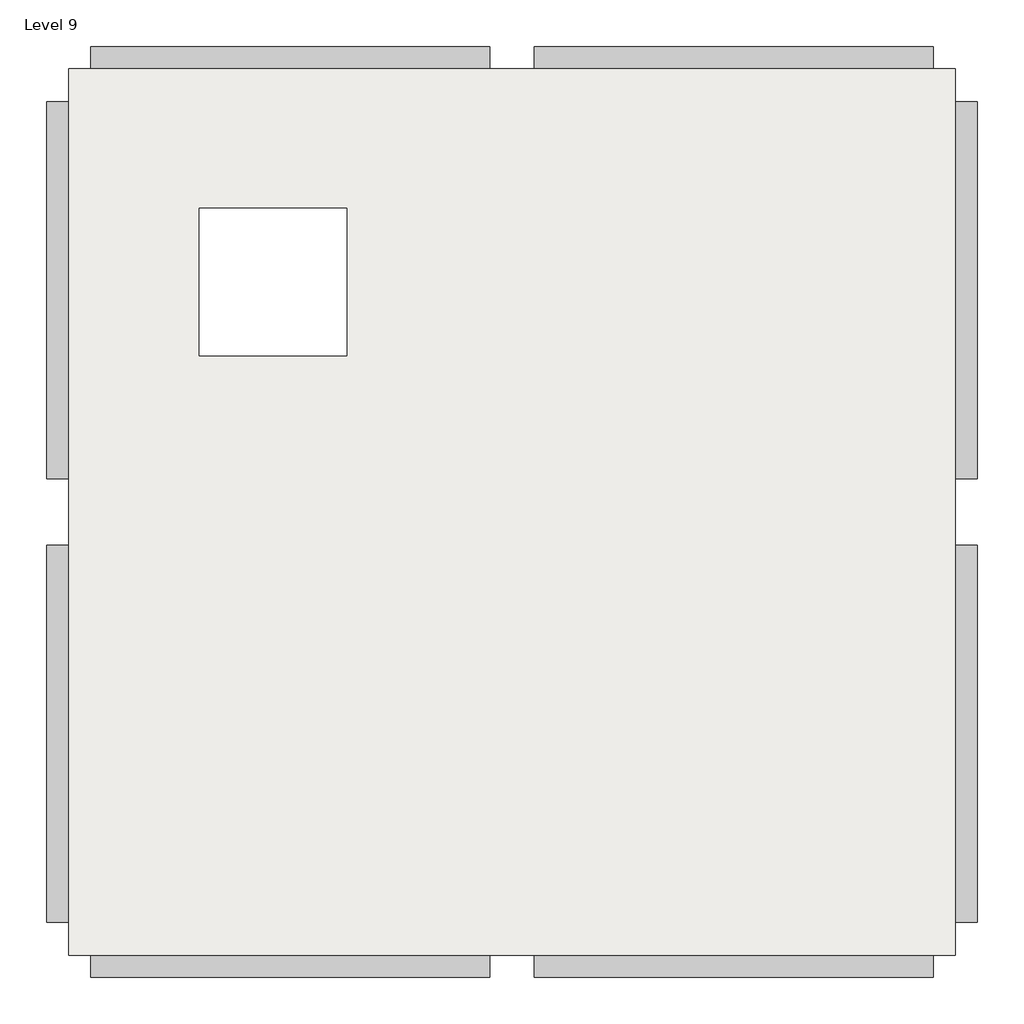
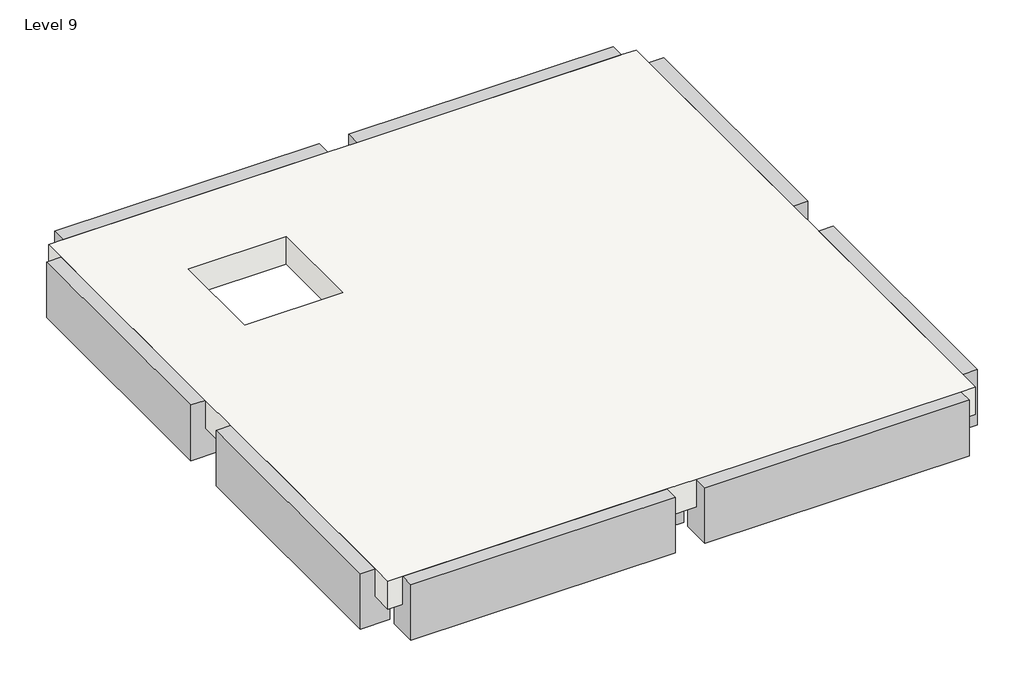
# One storey: 6 beams, 1 slab.
"""IFC4 building model written with IfcOpenShell, lengths in millimetres."""

from ifc_helpers import new_model, si_unit, frame, origin, place, context, project, spatial, polyline, outline, extrude, faceted_brep, element, save

model = new_model("IFC4")

# Units and contexts
model_context = context("Model", 3, world=origin())
ifc_project = project(units=[si_unit("LENGTHUNIT", "METRE", prefix="MILLI")], contexts=[model_context])

# Site, building, storey
site = spatial("IfcSite", under=ifc_project)
building = spatial("IfcBuilding", under=site)
storey = spatial("IfcBuildingStorey", under=building, Name="Level 9", Elevation=24000.0)

# Beams
placement = place(None, origin())
element("IfcBeam", 1, ObjectType="Concrete-Rectangular Beam : 300 x 600mm", at=placement, inside=storey, context=model_context, shape_type="SweptSolid", body=[
    extrude(outline(polyline([(526.3372902, 23400.0), (226.3372902, 23400.0), (226.3372902, 23700.0), (376.3372902, 23700.0), (376.3372902, 24000.0), (526.3372902, 24000.0), (526.3372902, 23400.0)])), frame((2068.7595868, 0.0, 0.0), z_axis=(1.0, 0.0, 0.0), x_axis=(0.0, 1.0, 0.0)), (0.0, 0.0, 1.0), 2700.0),
    extrude(outline(polyline([(526.3372902, 23400.0), (226.3372902, 23400.0), (226.3372902, 23700.0), (376.3372902, 23700.0), (376.3372902, 24000.0), (526.3372902, 24000.0), (526.3372902, 23400.0)])), frame((-931.2404132, 0.0, 0.0), z_axis=(1.0, 0.0, 0.0), x_axis=(0.0, 1.0, 0.0)), (0.0, 0.0, 1.0), 2700.0),
])
element("IfcBeam", 2, ObjectType="Concrete-Rectangular Beam : 300 x 600mm", at=placement, inside=storey, context=model_context, shape_type="SweptSolid", body=[
    extrude(outline(polyline([(23400.0, 5068.7595868), (24000.0, 5068.7595868), (24000.0, 4918.7595868), (23700.0, 4918.7595868), (23700.0, 4768.7595868), (23400.0, 4768.7595868), (23400.0, 5068.7595868)])), frame((0.0, -2398.6627098, 0.0), z_axis=(0.0, 1.0, 0.0), x_axis=(0.0, 0.0, 1.0)), (0.0, 0.0, 1.0), 2550.0),
    extrude(outline(polyline([(23400.0, 5068.7595868), (24000.0, 5068.7595868), (24000.0, 4918.7595868), (23700.0, 4918.7595868), (23700.0, 4768.7595868), (23400.0, 4768.7595868), (23400.0, 5068.7595868)])), frame((0.0, -5398.6627098, 0.0), z_axis=(0.0, 1.0, 0.0), x_axis=(0.0, 0.0, 1.0)), (0.0, 0.0, 1.0), 2550.0),
])
element("IfcBeam", 3, ObjectType="Concrete-Rectangular Beam : 300 x 600mm", at=placement, inside=storey, context=model_context, shape_type="SweptSolid", body=[
    extrude(outline(polyline([(-5773.6627098, 23400.0), (-5773.6627098, 24000.0), (-5623.6627098, 24000.0), (-5623.6627098, 23700.0), (-5473.6627098, 23700.0), (-5473.6627098, 23400.0), (-5773.6627098, 23400.0)])), frame((2068.7595868, 0.0, 0.0), z_axis=(1.0, 0.0, 0.0), x_axis=(0.0, 1.0, 0.0)), (0.0, 0.0, 1.0), 2700.0),
    extrude(outline(polyline([(-5773.6627098, 23400.0), (-5773.6627098, 24000.0), (-5623.6627098, 24000.0), (-5623.6627098, 23700.0), (-5473.6627098, 23700.0), (-5473.6627098, 23400.0), (-5773.6627098, 23400.0)])), frame((-931.2404132, 0.0, 0.0), z_axis=(1.0, 0.0, 0.0), x_axis=(0.0, 1.0, 0.0)), (0.0, 0.0, 1.0), 2700.0),
])
element("IfcBeam", 4, ObjectType="Concrete-Rectangular Beam : 300 x 600mm", at=placement, inside=storey, context=model_context, shape_type="SweptSolid", body=[
    extrude(outline(polyline([(24000.0, -1231.2404132), (23400.0, -1231.2404132), (23400.0, -931.2404132), (23700.0, -931.2404132), (23700.0, -1081.2404132), (24000.0, -1081.2404132), (24000.0, -1231.2404132)])), frame((0.0, -5398.6627098, 0.0), z_axis=(0.0, 1.0, 0.0), x_axis=(0.0, 0.0, 1.0)), (0.0, 0.0, 1.0), 2550.0),
    extrude(outline(polyline([(24000.0, -1231.2404132), (23400.0, -1231.2404132), (23400.0, -931.2404132), (23700.0, -931.2404132), (23700.0, -1081.2404132), (24000.0, -1081.2404132), (24000.0, -1231.2404132)])), frame((0.0, -2398.6627098, 0.0), z_axis=(0.0, 1.0, 0.0), x_axis=(0.0, 0.0, 1.0)), (0.0, 0.0, 1.0), 2550.0),
])
element("IfcBeam", 5, ObjectType="Concrete-Rectangular Beam : 300 x 600mm", at=placement, inside=storey, context=model_context, shape_type="SweptSolid", body=[
    extrude(outline(polyline([(2068.7595868, -5398.6627098), (1768.7595868, -5398.6627098), (1768.7595868, -2848.6627098), (2068.7595868, -2848.6627098), (2068.7595868, -5398.6627098)])), frame((0.0, 0.0, 23400.0), z_axis=(0.0, 0.0, 1.0), x_axis=(1.0, 0.0, 0.0)), (0.0, 0.0, 1.0), 300.0),
    extrude(outline(polyline([(1768.7595868, 151.3372902), (2068.7595868, 151.3372902), (2068.7595868, -2398.6627098), (1768.7595868, -2398.6627098), (1768.7595868, 151.3372902)])), frame((0.0, 0.0, 23400.0), z_axis=(0.0, 0.0, 1.0), x_axis=(1.0, 0.0, 0.0)), (0.0, 0.0, 1.0), 300.0),
])
element("IfcBeam", 6, ObjectType="Concrete-Rectangular Beam : 300 x 600mm", at=placement, inside=storey, context=model_context, shape_type="SweptSolid", body=[
    extrude(outline(polyline([(4768.7595868, -2473.6627098), (4768.7595868, -2773.6627098), (2068.7595868, -2773.6627098), (2068.7595868, -2473.6627098), (4768.7595868, -2473.6627098)])), frame((0.0, 0.0, 23400.0), z_axis=(0.0, 0.0, 1.0), x_axis=(1.0, 0.0, 0.0)), (0.0, 0.0, 1.0), 300.0),
    extrude(outline(polyline([(-931.2404132, -2773.6627098), (-931.2404132, -2473.6627098), (1768.7595868, -2473.6627098), (1768.7595868, -2773.6627098), (-931.2404132, -2773.6627098)])), frame((0.0, 0.0, 23400.0), z_axis=(0.0, 0.0, 1.0), x_axis=(1.0, 0.0, 0.0)), (0.0, 0.0, 1.0), 300.0),
])

# Slab
element("IfcSlab", 7, ObjectType="Generic 300mm", at=placement, inside=storey, context=model_context, shape_type="Brep", body=[
    faceted_brep([(4918.7595868, 376.3372902, 23700.0), (4918.7595868, 151.3372902, 23700.0), (4918.7595868, -2398.6627098, 23700.0), (4918.7595868, -2848.6627098, 23700.0), (4918.7595868, -5398.6627098, 23700.0), (4918.7595868, -5623.6627098, 23700.0), (4768.7595868, -5623.6627098, 23700.0), (2068.7595868, -5623.6627098, 23700.0), (1768.7595868, -5623.6627098, 23700.0), (-931.2404132, -5623.6627098, 23700.0), (-1081.2404132, -5623.6627098, 23700.0), (-1081.2404132, -5398.6627098, 23700.0), (-1081.2404132, -2848.6627098, 23700.0), (-1081.2404132, -2398.6627098, 23700.0), (-1081.2404132, 151.3372902, 23700.0), (-1081.2404132, 376.3372902, 23700.0), (-931.2404132, 376.3372902, 23700.0), (1768.7595868, 376.3372902, 23700.0), (2068.7595868, 376.3372902, 23700.0), (4768.7595868, 376.3372902, 23700.0), (-198.5229478, -1566.5574371, 23700.0), (801.4770522, -1566.5574371, 23700.0), (801.4770522, -566.5574371, 23700.0), (-198.5229478, -566.5574371, 23700.0), (4918.7595868, -5623.6627098, 24000.0), (4918.7595868, -5398.6627098, 24000.0), (4918.7595868, -2848.6627098, 24000.0), (4918.7595868, -2398.6627098, 24000.0), (4918.7595868, 151.3372902, 24000.0), (4918.7595868, 376.3372902, 24000.0), (4768.7595868, 376.3372902, 24000.0), (2068.7595868, 376.3372902, 24000.0), (1768.7595868, 376.3372902, 24000.0), (-931.2404132, 376.3372902, 24000.0), (-1081.2404132, 376.3372902, 24000.0), (-1081.2404132, 151.3372902, 24000.0), (-1081.2404132, -2398.6627098, 24000.0), (-1081.2404132, -2848.6627098, 24000.0), (-1081.2404132, -5398.6627098, 24000.0), (-1081.2404132, -5623.6627098, 24000.0), (-931.2404132, -5623.6627098, 24000.0), (1768.7595868, -5623.6627098, 24000.0), (2068.7595868, -5623.6627098, 24000.0), (4768.7595868, -5623.6627098, 24000.0), (801.4770522, -1566.5574371, 24000.0), (-198.5229478, -1566.5574371, 24000.0), (-198.5229478, -566.5574371, 24000.0), (801.4770522, -566.5574371, 24000.0)], [[[0, 1, 2, 3, 4, 5, 6, 7, 8, 9, 10, 11, 12, 13, 14, 15, 16, 17, 18, 19], [20, 21, 22, 23]], [[24, 25, 26, 27, 28, 29, 30, 31, 32, 33, 34, 35, 36, 37, 38, 39, 40, 41, 42, 43], [44, 45, 46, 47]], [[5, 4, 3, 2, 1, 0, 29, 28, 27, 26, 25, 24]], [[10, 9, 8, 7, 6, 5, 24, 43, 42, 41, 40, 39]], [[15, 14, 13, 12, 11, 10, 39, 38, 37, 36, 35, 34]], [[0, 19, 18, 17, 16, 15, 34, 33, 32, 31, 30, 29]], [[20, 45, 44, 21]], [[21, 44, 47, 22]], [[22, 47, 46, 23]], [[45, 20, 23, 46]]]),
])

save(model, "model.ifc")

# Revit data of these elements
# Type "Concrete-Rectangular Beam : 300 x 600mm"
#   Length [instance default] = 1.524 m
#   b = 0.3 m
#   h = 0.6 m
#   Structural Material [instance default] = Concrete, Cast-in-Place gray
#   Assembly Code = ""
# Type "Generic 300mm"
#   Function = 0
#   Layers, outside or top first: 0.3 m no material (function 1)
# Elements 1, 2, 3, 4, 5, 6 (IfcBeam, "Concrete-Rectangular Beam : 300 x 600mm")
#   Structural Material = Concrete, Cast-in-Place gray
#   Phase Created = New Construction
#   Materials on its faces: "Concrete, Cast-in-Place gray"
# Element 7 (IfcSlab, "Generic 300mm")
#   Height Offset From Level = 0 m
#   built-in parameter 1001954 = 1
#   Phase Created = New Construction
#   Materials on its faces: "Default Floor"
# Materials
#   "Concrete, Cast-in-Place gray": class "Concrete", colour RGB 192 192 192, transparency 0, Description = "Cast-in-place concrete", Cost = 0
#   "Default Floor": colour RGB 127 127 127, transparency 0, Cost = 0
